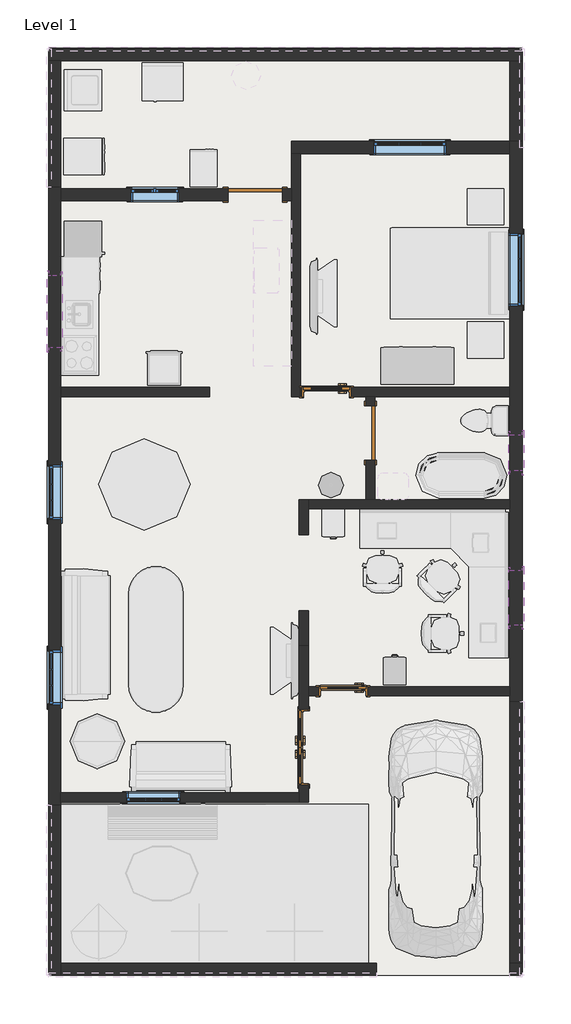
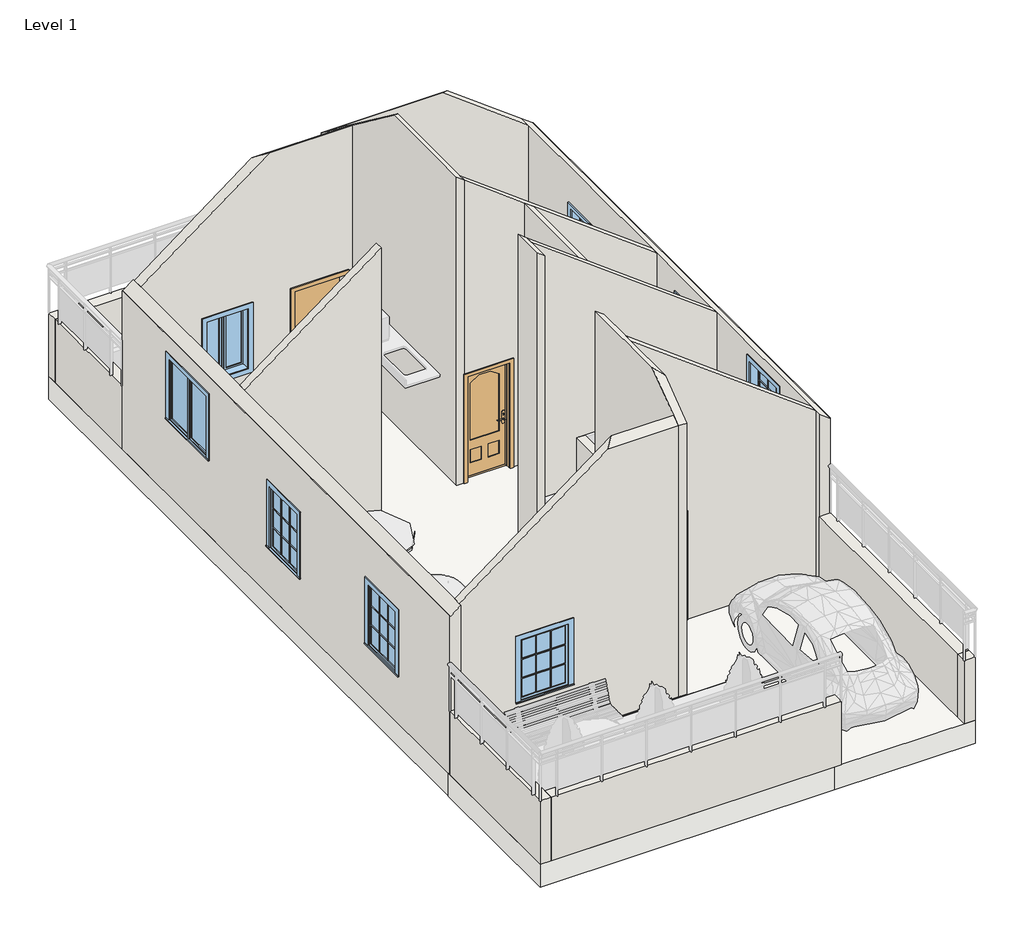
# One storey, part 1 of 3: 21 walls, 9 windows, 5 doors, 2 slabs.
"""IFC4 building model written with IfcOpenShell, lengths in millimetres."""

from ifc_helpers import new_model, si_unit, frame, origin, origin_with_axes, place, context, project, spatial, polyline, outline, extrude, faceted_brep, transform, mapped, element, save
from components import door_14b9be53, door_3efe7946, door_686f89d2, door_54dd4da4, window_29c06734, window_5c190c7e, window_99fc0ff6, window_bb17773d, window_0862ab64, window_e41d21a6

model = new_model("IFC4")

# Units and contexts
model_context = context("Model", 3, world=origin())
ifc_project = project(units=[si_unit("LENGTHUNIT", "METRE", prefix="MILLI")], contexts=[model_context])

# Site, building, storey
site = spatial("IfcSite", under=ifc_project)
building = spatial("IfcBuilding", under=site)
storey = spatial("IfcBuildingStorey", under=building, Name="Level 1", Elevation=0.0)

# Doors
placement = place(None, origin())
door_shape = door_14b9be53(model_context)
element("IfcDoor", 1, ObjectType="30\" x 80\"", at=placement, inside=storey, context=model_context, shape_type="MappedRepresentation", body=[
    mapped(door_shape, transform((-3257.4124913, 1119.1144299, 0.0), x_axis=(1.0, 0.0, 0.0), y_axis=(0.0, 1.0, 0.0), z_axis=(0.0, 0.0, 1.0))),
])
element("IfcDoor", 2, ObjectType="30\" x 80\"", at=placement, inside=storey, context=model_context, shape_type="MappedRepresentation", body=[
    mapped(door_shape, transform((-3536.8124913, 6122.9144299, 0.0), x_axis=(1.0, 0.0, 0.0), y_axis=(0.0, 1.0, 0.0), z_axis=(0.0, 0.0, 1.0))),
])
door_2_shape = door_3efe7946(model_context)
element("IfcDoor", 3, ObjectType="Door-Exterior-Double-Full Glass-Wood_Clad : 48\" x 80\"", at=placement, inside=storey, context=model_context, shape_type="MappedRepresentation", body=[
    mapped(door_2_shape, transform((-3920.9874913, 176.1394299, 0.0), x_axis=(0.0, 1.0, 0.0), y_axis=(-1.0, 0.0, 0.0), z_axis=(0.0, 0.0, 1.0))),
])
door_3_shape = door_686f89d2(model_context)
element("IfcDoor", 4, ObjectType="Single-Flush : 36\" x 84\"", at=placement, inside=storey, context=model_context, shape_type="MappedRepresentation", body=[
    mapped(door_3_shape, transform((-2800.2124913, 5433.9394299, 0.0), x_axis=(0.0, 1.0, 0.0), y_axis=(-1.0, 0.0, 0.0), z_axis=(0.0, 0.0, 1.0))),
])
door_4_shape = door_54dd4da4(model_context)
element("IfcDoor", 5, ObjectType="Single-Flush : 36\" x 84\"", at=placement, inside=storey, context=model_context, shape_type="MappedRepresentation", body=[
    mapped(door_4_shape, transform((-4730.6124913, 9421.7394299, 0.0), x_axis=(1.0, 0.0, 0.0), y_axis=(0.0, 1.0, 0.0), z_axis=(0.0, 0.0, 1.0))),
])

# Slabs
element("IfcSlab", 6, ObjectType="Steel Bar Joist 14\" - VCT on Concrete", at=placement, inside=storey, context=model_context, shape_type="SweptSolid", body=[
    extrude(outline(polyline([(-260.2124913, 11866.4894299), (-260.2124913, -3633.8605701), (-2825.6124913, -3633.8605701), (-2825.6124913, -763.6605701), (-8185.0124913, -763.6605701), (-8185.0124913, 11866.4894299), (-260.2124913, 11866.4894299)])), frame((0.0, 0.0, -441.325), z_axis=(0.0, 0.0, 1.0), x_axis=(1.0, 0.0, 0.0)), (0.0, 0.0, 1.0), 441.325),
])
element("IfcSlab", 7, ObjectType="Steel Bar Joist 14\" - VCT on Concrete", at=placement, inside=storey, context=model_context, shape_type="SweptSolid", body=[
    extrude(outline(polyline([(-8185.0124913, -738.2605701), (-7981.8124913, -738.2605701), (-7981.8124913, -3430.6605701), (-2825.6124913, -3430.6605701), (-2825.6124913, -3633.8605701), (-8185.0124913, -3633.8605701), (-8185.0124913, -738.2605701)])), frame((0.0, 0.0, -441.325), z_axis=(0.0, 0.0, 1.0), x_axis=(1.0, 0.0, 0.0)), (0.0, 0.0, 1.0), 441.325),
])

# Walls
element("IfcWall", 8, ObjectType="Generic - 8\"", at=placement, inside=storey, context=model_context, shape_type="Brep", body=[
    faceted_brep([(-8185.0124913, 11656.9394299, 0.0), (-7981.8124913, 11656.9394299, 0.0), (-463.4124913, 11656.9394299, 0.0), (-260.2124913, 11656.9394299, 0.0), (-260.2124913, 11656.9394299, 1219.2), (-463.4124913, 11656.9394299, 1219.2), (-7981.8124913, 11656.9394299, 1219.2), (-8185.0124913, 11656.9394299, 1219.2), (-8185.0124913, 11860.1394299, 0.0), (-8185.0124913, 11860.1394299, 1219.2), (-260.2124913, 11860.1394299, 1219.2), (-260.2124913, 11860.1394299, 0.0)], [[[0, 1, 2, 3, 4, 5, 6, 7]], [[8, 9, 10, 11]], [[3, 2, 1, 0, 8, 11]], [[7, 6, 5, 4, 10, 9]], [[0, 7, 9, 8]], [[4, 3, 11, 10]]]),
])
element("IfcWall", 9, ObjectType="Generic - 8\"", at=placement, inside=storey, context=model_context, shape_type="SweptSolid", body=[
    extrude(outline(polyline([(-8185.0124913, 9548.7394299), (-8185.0124913, 11656.9394299), (-7981.8124913, 11656.9394299), (-7981.8124913, 9548.7394299), (-8185.0124913, 9548.7394299)])), origin_with_axes(), (0.0, 0.0, 1.0), 1219.2),
])
element("IfcWall", 10, ObjectType="Generic - 8\"", at=placement, inside=storey, context=model_context, shape_type="SweptSolid", body=[
    extrude(outline(polyline([(-2698.6124913, -3633.8605701), (-7981.8124913, -3633.8605701), (-7981.8124913, -3430.6605701), (-2698.6124913, -3430.6605701), (-2698.6124913, -3633.8605701)])), origin_with_axes(), (0.0, 0.0, 1.0), 1219.2),
])
element("IfcWall", 11, ObjectType="Generic - 8\"", at=placement, inside=storey, context=model_context, shape_type="SweptSolid", body=[
    extrude(outline(polyline([(-260.2124913, 938.1394299), (-260.2124913, -3430.6605701), (-463.4124913, -3430.6605701), (-463.4124913, 938.1394299), (-260.2124913, 938.1394299)])), origin_with_axes(), (0.0, 0.0, 1.0), 1219.2),
])
element("IfcWall", 12, ObjectType="Generic - 8\"", at=placement, inside=storey, context=model_context, shape_type="Brep", body=[
    faceted_brep([(-463.4124913, 10310.7394299, 3193.25625), (-463.4124913, 10310.7394299, 0.0), (-4121.0124913, 10310.7394299, 0.0), (-4121.0124913, 10310.7394299, 4210.05), (-1819.1374913, 10310.7394299, 4210.05), (-1530.2124913, 10310.7394299, 1828.8), (-2749.4124913, 10310.7394299, 1828.8), (-2749.4124913, 10310.7394299, 304.8), (-1530.2124913, 10310.7394299, 304.8), (-463.4124913, 10107.5394299, 0.0), (-463.4124913, 10107.5394299, 3193.25625), (-2022.3374913, 10107.5394299, 4362.45), (-3968.6124913, 10107.5394299, 4362.45), (-4121.0124913, 10107.5394299, 4362.45), (-4121.0124913, 10107.5394299, 0.0), (-3968.6124913, 10107.5394299, 0.0), (-1530.2124913, 10107.5394299, 1828.8), (-1530.2124913, 10107.5394299, 304.8), (-2749.4124913, 10107.5394299, 304.8), (-2749.4124913, 10107.5394299, 1828.8)], [[[0, 1, 2, 3, 4], [5, 6, 7, 8]], [[9, 10, 11, 12, 13, 14, 15], [16, 17, 18, 19]], [[2, 1, 9, 15, 14]], [[3, 2, 14, 13]], [[0, 10, 9, 1]], [[0, 4, 11, 10]], [[4, 3, 13, 12, 11]], [[17, 16, 5, 8]], [[18, 17, 8, 7]], [[19, 18, 7, 6]], [[16, 19, 6, 5]]]),
])
element("IfcWall", 13, ObjectType="Generic - 8\"", at=placement, inside=storey, context=model_context, shape_type="Brep", body=[
    faceted_brep([(-4273.4124913, 9320.1394299, 2133.6), (-4273.4124913, 9320.1394299, 0.0), (-4121.0124913, 9320.1394299, 0.0), (-4121.0124913, 9320.1394299, 4953.0), (-5632.3124913, 9320.1394299, 4953.0), (-7981.8124913, 9320.1394299, 3190.875), (-7981.8124913, 9320.1394299, 0.0), (-5187.8124913, 9320.1394299, 0.0), (-5187.8124913, 9320.1394299, 2133.6), (-6000.6124913, 9320.1394299, 2133.6), (-6000.6124913, 9320.1394299, 914.4), (-6813.4124913, 9320.1394299, 914.4), (-6813.4124913, 9320.1394299, 2133.6), (-4121.0124913, 9523.3394299, 0.0), (-4273.4124913, 9523.3394299, 0.0), (-4273.4124913, 9523.3394299, 2133.6), (-5187.8124913, 9523.3394299, 2133.6), (-5187.8124913, 9523.3394299, 0.0), (-7981.8124913, 9523.3394299, 0.0), (-7981.8124913, 9523.3394299, 3190.875), (-5835.5124913, 9523.3394299, 4800.6), (-4121.0124913, 9523.3394299, 4800.6), (-6000.6124913, 9523.3394299, 2133.6), (-6813.4124913, 9523.3394299, 2133.6), (-6813.4124913, 9523.3394299, 914.4), (-6000.6124913, 9523.3394299, 914.4)], [[[0, 1, 2, 3, 4, 5, 6, 7, 8], [9, 10, 11, 12]], [[13, 14, 15, 16, 17, 18, 19, 20, 21], [22, 23, 24, 25]], [[7, 6, 18, 17]], [[2, 1, 14, 13]], [[6, 5, 19, 18]], [[3, 2, 13, 21]], [[5, 4, 20, 19]], [[4, 3, 21, 20]], [[15, 14, 1, 0]], [[16, 15, 0, 8]], [[17, 16, 8, 7]], [[10, 9, 22, 25]], [[11, 10, 25, 24]], [[12, 11, 24, 23]], [[9, 12, 23, 22]]]),
])
element("IfcWall", 14, ObjectType="Generic - 8\"", at=placement, inside=storey, context=model_context, shape_type="Brep", body=[
    faceted_brep([(-8185.0124913, -789.0605701, 0.0), (-8185.0124913, -3633.8605701, 0.0), (-8185.0124913, -3633.8605701, 1219.2), (-8185.0124913, -789.0605701, 1219.2), (-7981.8124913, -789.0605701, 0.0), (-7981.8124913, -789.0605701, 1219.2), (-7981.8124913, -3430.6605701, 1219.2), (-7981.8124913, -3633.8605701, 1219.2), (-7981.8124913, -3633.8605701, 0.0), (-7981.8124913, -3430.6605701, 0.0)], [[[0, 1, 2, 3]], [[4, 5, 6, 7, 8, 9]], [[1, 0, 4, 9, 8]], [[3, 2, 7, 6, 5]], [[0, 3, 5, 4]], [[2, 1, 8, 7]]]),
])
element("IfcWall", 15, ObjectType="Generic - 8\"", at=placement, inside=storey, context=model_context, shape_type="SweptSolid", body=[
    extrude(outline(polyline([(-260.2124913, -3633.8605701), (-463.4124913, -3633.8605701), (-463.4124913, -3430.6605701), (-260.2124913, -3430.6605701), (-260.2124913, -3633.8605701)])), origin_with_axes(), (0.0, 0.0, 1.0), 1219.2),
])
element("IfcWall", 16, ObjectType="Generic - 8\"", at=placement, inside=storey, context=model_context, shape_type="Brep", body=[
    faceted_brep([(-260.2124913, 938.1394299, 0.0), (-260.2124913, 10310.7394299, 0.0), (-260.2124913, 10310.7394299, 1219.2), (-260.2124913, 10310.7394299, 3048.0), (-260.2124913, 938.1394299, 3048.0), (-260.2124913, 938.1394299, 1219.2), (-260.2124913, 2220.8394299, 2927.35), (-260.2124913, 3135.2394299, 2927.35), (-260.2124913, 3135.2394299, 1708.15), (-260.2124913, 2220.8394299, 1708.15), (-260.2124913, 7554.8394299, 2438.4), (-260.2124913, 8774.0394299, 2438.4), (-260.2124913, 8774.0394299, 914.4), (-260.2124913, 7554.8394299, 914.4), (-260.2124913, 4798.9394299, 2768.6), (-260.2124913, 5408.5394299, 2768.6), (-260.2124913, 5408.5394299, 2159.0), (-260.2124913, 4798.9394299, 2159.0), (-463.4124913, 938.1394299, 0.0), (-463.4124913, 938.1394299, 1219.2), (-463.4124913, 938.1394299, 3193.25625), (-463.4124913, 1039.7394299, 3193.25625), (-463.4124913, 1192.1394299, 3193.25625), (-463.4124913, 4163.9394299, 3193.25625), (-463.4124913, 4316.3394299, 3193.25625), (-463.4124913, 6043.5394299, 3193.25625), (-463.4124913, 6195.9394299, 3193.25625), (-463.4124913, 10107.5394299, 3193.25625), (-463.4124913, 10310.7394299, 3193.25625), (-463.4124913, 10310.7394299, 1219.2), (-463.4124913, 10310.7394299, 0.0), (-463.4124913, 10107.5394299, 0.0), (-463.4124913, 6195.9394299, 0.0), (-463.4124913, 6043.5394299, 0.0), (-463.4124913, 4316.3394299, 0.0), (-463.4124913, 4163.9394299, 0.0), (-463.4124913, 1192.1394299, 0.0), (-463.4124913, 1039.7394299, 0.0), (-463.4124913, 2220.8394299, 2927.35), (-463.4124913, 2220.8394299, 1708.15), (-463.4124913, 3135.2394299, 1708.15), (-463.4124913, 3135.2394299, 2927.35), (-463.4124913, 7554.8394299, 2438.4), (-463.4124913, 7554.8394299, 914.4), (-463.4124913, 8774.0394299, 914.4), (-463.4124913, 8774.0394299, 2438.4), (-463.4124913, 4798.9394299, 2768.6), (-463.4124913, 4798.9394299, 2159.0), (-463.4124913, 5408.5394299, 2159.0), (-463.4124913, 5408.5394299, 2768.6), (-269.7374913, 938.1394299, 3048.0), (-269.7374913, 10310.7394299, 3048.0)], [[[0, 1, 2, 3, 4, 5], [6, 7, 8, 9], [10, 11, 12, 13], [14, 15, 16, 17]], [[18, 19, 20, 21, 22, 23, 24, 25, 26, 27, 28, 29, 30, 31, 32, 33, 34, 35, 36, 37], [38, 39, 40, 41], [42, 43, 44, 45], [46, 47, 48, 49]], [[1, 0, 18, 37, 36, 35, 34, 33, 32, 31, 30]], [[0, 5, 4, 50, 20, 19, 18]], [[1, 30, 29, 28, 51, 3, 2]], [[4, 3, 51, 50]], [[51, 28, 27, 26, 25, 24, 23, 22, 21, 20, 50]], [[39, 38, 6, 9]], [[40, 39, 9, 8]], [[41, 40, 8, 7]], [[38, 41, 7, 6]], [[43, 42, 10, 13]], [[44, 43, 13, 12]], [[45, 44, 12, 11]], [[42, 45, 11, 10]], [[47, 46, 14, 17]], [[48, 47, 17, 16]], [[49, 48, 16, 15]], [[46, 49, 15, 14]]]),
])
element("IfcWall", 17, ObjectType="Generic - 8\"", at=placement, inside=storey, context=model_context, shape_type="Brep", body=[
    faceted_brep([(-8185.0124913, 9548.7394299, 0.0), (-8185.0124913, -789.0605701, 0.0), (-8185.0124913, -789.0605701, 1219.2), (-8185.0124913, -789.0605701, 3048.0), (-8185.0124913, 9548.7394299, 3048.0), (-8185.0124913, 9548.7394299, 1219.2), (-8185.0124913, 1801.7394299, 2133.6), (-8185.0124913, 887.3394299, 2133.6), (-8185.0124913, 887.3394299, 914.4), (-8185.0124913, 1801.7394299, 914.4), (-8185.0124913, 4900.5394299, 2133.6), (-8185.0124913, 3986.1394299, 2133.6), (-8185.0124913, 3986.1394299, 914.4), (-8185.0124913, 4900.5394299, 914.4), (-8185.0124913, 8075.5394299, 2667.0), (-8185.0124913, 6856.3394299, 2667.0), (-8185.0124913, 6856.3394299, 1447.8), (-8185.0124913, 8075.5394299, 1447.8), (-7981.8124913, 9548.7394299, 0.0), (-7981.8124913, 9548.7394299, 1219.2), (-7981.8124913, 9548.7394299, 3190.875), (-7981.8124913, 9523.3394299, 3190.875), (-7981.8124913, 9320.1394299, 3190.875), (-7981.8124913, 6195.9394299, 3190.875), (-7981.8124913, 6043.5394299, 3190.875), (-7981.8124913, -585.8605701, 3190.875), (-7981.8124913, -738.2605701, 3190.875), (-7981.8124913, -789.0605701, 3190.875), (-7981.8124913, -789.0605701, 1219.2), (-7981.8124913, -789.0605701, 0.0), (-7981.8124913, -738.2605701, 0.0), (-7981.8124913, -585.8605701, 0.0), (-7981.8124913, 6043.5394299, 0.0), (-7981.8124913, 6195.9394299, 0.0), (-7981.8124913, 9320.1394299, 0.0), (-7981.8124913, 9523.3394299, 0.0), (-7981.8124913, 1801.7394299, 2133.6), (-7981.8124913, 1801.7394299, 914.4), (-7981.8124913, 887.3394299, 914.4), (-7981.8124913, 887.3394299, 2133.6), (-7981.8124913, 4900.5394299, 2133.6), (-7981.8124913, 4900.5394299, 914.4), (-7981.8124913, 3986.1394299, 914.4), (-7981.8124913, 3986.1394299, 2133.6), (-7981.8124913, 8075.5394299, 2667.0), (-7981.8124913, 8075.5394299, 1447.8), (-7981.8124913, 6856.3394299, 1447.8), (-7981.8124913, 6856.3394299, 2667.0), (-8172.3124913, -789.0605701, 3048.0), (-8172.3124913, 9548.7394299, 3048.0)], [[[0, 1, 2, 3, 4, 5], [6, 7, 8, 9], [10, 11, 12, 13], [14, 15, 16, 17]], [[18, 19, 20, 21, 22, 23, 24, 25, 26, 27, 28, 29, 30, 31, 32, 33, 34, 35], [36, 37, 38, 39], [40, 41, 42, 43], [44, 45, 46, 47]], [[1, 0, 18, 35, 34, 33, 32, 31, 30, 29]], [[3, 2, 1, 29, 28, 27, 48]], [[0, 5, 4, 49, 20, 19, 18]], [[4, 3, 48, 49]], [[48, 27, 26, 25, 24, 23, 22, 21, 20, 49]], [[37, 36, 6, 9]], [[38, 37, 9, 8]], [[39, 38, 8, 7]], [[36, 39, 7, 6]], [[41, 40, 10, 13]], [[42, 41, 13, 12]], [[43, 42, 12, 11]], [[40, 43, 11, 10]], [[45, 44, 14, 17]], [[46, 45, 17, 16]], [[47, 46, 16, 15]], [[44, 47, 15, 14]]]),
])
element("IfcWall", 18, ObjectType="Generic - 8\"", at=placement, inside=storey, context=model_context, shape_type="SweptSolid", body=[
    extrude(outline(polyline([(-260.2124913, 11656.9394299), (-260.2124913, 10310.7394299), (-463.4124913, 10310.7394299), (-463.4124913, 11656.9394299), (-260.2124913, 11656.9394299)])), origin_with_axes(), (0.0, 0.0, 1.0), 1219.2),
])
element("IfcWall", 19, ObjectType="INNER WALL", at=placement, inside=storey, context=model_context, shape_type="Brep", body=[
    faceted_brep([(-4121.0124913, 10107.5394299, 0.0), (-4121.0124913, 9523.3394299, 0.0), (-4121.0124913, 9320.1394299, 0.0), (-4121.0124913, 6043.5394299, 0.0), (-4121.0124913, 6043.5394299, 5936.45625), (-4121.0124913, 8008.8644299, 5936.45625), (-4121.0124913, 9320.1394299, 4953.0), (-4121.0124913, 9523.3394299, 4800.6), (-4121.0124913, 10107.5394299, 4362.45), (-3968.6124913, 10107.5394299, 0.0), (-3968.6124913, 10107.5394299, 4362.45), (-3968.6124913, 8161.2644299, 5822.15625), (-3968.6124913, 6195.9394299, 5822.15625), (-3968.6124913, 6043.5394299, 5822.15625), (-3968.6124913, 6043.5394299, 0.0), (-3968.6124913, 6195.9394299, 0.0)], [[[0, 1, 2, 3, 4, 5, 6, 7, 8]], [[9, 10, 11, 12, 13, 14, 15]], [[3, 2, 1, 0, 9, 15, 14]], [[0, 8, 10, 9]], [[4, 3, 14, 13]], [[8, 7, 6, 5, 11, 10]], [[5, 4, 13, 12, 11]]]),
])
element("IfcWall", 20, ObjectType="INNER WALL", at=placement, inside=storey, context=model_context, shape_type="Brep", body=[
    faceted_brep([(-463.4124913, 6195.9394299, 3193.25625), (-463.4124913, 6195.9394299, 0.0), (-3130.4124913, 6195.9394299, 0.0), (-3130.4124913, 6195.9394299, 2057.4), (-3943.2124913, 6195.9394299, 2057.4), (-3943.2124913, 6195.9394299, 0.0), (-3968.6124913, 6195.9394299, 0.0), (-3968.6124913, 6195.9394299, 5822.15625), (-463.4124913, 6043.5394299, 0.0), (-463.4124913, 6043.5394299, 3193.25625), (-2724.0124913, 6043.5394299, 4888.70625), (-2876.4124913, 6043.5394299, 5003.00625), (-3968.6124913, 6043.5394299, 5822.15625), (-3968.6124913, 6043.5394299, 0.0), (-3943.2124913, 6043.5394299, 0.0), (-3943.2124913, 6043.5394299, 2057.4), (-3130.4124913, 6043.5394299, 2057.4), (-3130.4124913, 6043.5394299, 0.0), (-2876.4124913, 6043.5394299, 0.0), (-2724.0124913, 6043.5394299, 0.0)], [[[0, 1, 2, 3, 4, 5, 6, 7]], [[8, 9, 10, 11, 12, 13, 14, 15, 16, 17, 18, 19]], [[1, 8, 19, 18, 17, 2]], [[13, 6, 5, 14]], [[1, 0, 9, 8]], [[7, 6, 13, 12]], [[0, 7, 12, 11, 10, 9]], [[16, 3, 2, 17]], [[3, 16, 15, 4]], [[4, 15, 14, 5]]]),
])
element("IfcWall", 21, ObjectType="INNER WALL", at=placement, inside=storey, context=model_context, shape_type="Brep", body=[
    faceted_brep([(-463.4124913, 4316.3394299, 0.0), (-2724.0124913, 4316.3394299, 0.0), (-2876.4124913, 4316.3394299, 0.0), (-3841.6124913, 4316.3394299, 0.0), (-3841.6124913, 4316.3394299, 5726.90625), (-2876.4124913, 4316.3394299, 5003.00625), (-2724.0124913, 4316.3394299, 4888.70625), (-463.4124913, 4316.3394299, 3193.25625), (-463.4124913, 4163.9394299, 0.0), (-463.4124913, 4163.9394299, 3193.25625), (-3841.6124913, 4163.9394299, 5726.90625), (-3841.6124913, 4163.9394299, 0.0)], [[[0, 1, 2, 3, 4, 5, 6, 7]], [[8, 9, 10, 11]], [[3, 2, 1, 0, 8, 11]], [[0, 7, 9, 8]], [[4, 3, 11, 10]], [[7, 6, 5, 4, 10, 9]]]),
])
element("IfcWall", 22, ObjectType="INNER WALL", at=placement, inside=storey, context=model_context, shape_type="SweptSolid", body=[
    extrude(outline(polyline([(0.0, -463.4124913), (3193.25625, -463.4124913), (5726.90625, -3841.6124913), (0.0, -3841.6124913), (0.0, -3663.8124913), (2057.4, -3663.8124913), (2057.4, -2851.0124913), (0.0, -2851.0124913), (0.0, -463.4124913)])), frame((0.0, 1039.7394299, 0.0), z_axis=(0.0, 1.0, 0.0), x_axis=(0.0, 0.0, 1.0)), (0.0, 0.0, 1.0), 152.4),
])
element("IfcWall", 23, ObjectType="INNER WALL", at=placement, inside=storey, context=model_context, shape_type="Brep", body=[
    faceted_brep([(-3994.0124913, -585.8605701, 0.0), (-7981.8124913, -585.8605701, 0.0), (-7981.8124913, -585.8605701, 3190.875), (-5127.4874913, -585.8605701, 5331.61875), (-3994.0124913, -585.8605701, 5331.61875), (-6889.6124913, -585.8605701, 2133.6), (-6889.6124913, -585.8605701, 914.4), (-5975.2124913, -585.8605701, 914.4), (-5975.2124913, -585.8605701, 2133.6), (-3994.0124913, -738.2605701, 0.0), (-3994.0124913, -738.2605701, 5217.31875), (-5279.8874913, -738.2605701, 5217.31875), (-7981.8124913, -738.2605701, 3190.875), (-7981.8124913, -738.2605701, 0.0), (-6889.6124913, -738.2605701, 2133.6), (-5975.2124913, -738.2605701, 2133.6), (-5975.2124913, -738.2605701, 914.4), (-6889.6124913, -738.2605701, 914.4)], [[[0, 1, 2, 3, 4], [5, 6, 7, 8]], [[9, 10, 11, 12, 13], [14, 15, 16, 17]], [[1, 0, 9, 13]], [[2, 1, 13, 12]], [[0, 4, 10, 9]], [[4, 3, 11, 10]], [[3, 2, 12, 11]], [[6, 5, 14, 17]], [[7, 6, 17, 16]], [[8, 7, 16, 15]], [[5, 8, 15, 14]]]),
])
element("IfcWall", 24, ObjectType="INNER WALL", at=placement, inside=storey, context=model_context, shape_type="SweptSolid", body=[
    extrude(outline(polyline([(0.0, -5492.6124913), (5057.775, -5492.6124913), (3190.875, -7981.8124913), (0.0, -7981.8124913), (0.0, -5492.6124913)])), frame((0.0, 6043.5394299, 0.0), z_axis=(0.0, 1.0, 0.0), x_axis=(0.0, 0.0, 1.0)), (0.0, 0.0, 1.0), 152.4),
])
element("IfcWall", 25, ObjectType="INNER WALL", at=placement, inside=storey, context=model_context, shape_type="Brep", body=[
    faceted_brep([(-3994.0124913, 1877.9394299, 5841.20625), (-3994.0124913, 1877.9394299, 3048.0), (-3994.0124913, 1877.9394299, 0.0), (-3994.0124913, 811.1394299, 0.0), (-3994.0124913, 811.1394299, 2057.4), (-3994.0124913, -458.8605701, 2057.4), (-3994.0124913, -458.8605701, 0.0), (-3994.0124913, -585.8605701, 0.0), (-3994.0124913, -738.2605701, 0.0), (-3994.0124913, -738.2605701, 5217.31875), (-3994.0124913, -585.8605701, 5331.61875), (-3994.0124913, 93.5894299, 5841.20625), (-3841.6124913, 1877.9394299, 0.0), (-3841.6124913, 1877.9394299, 3048.0), (-3841.6124913, 1877.9394299, 5726.90625), (-3841.6124913, 1192.1394299, 5726.90625), (-3841.6124913, 1039.7394299, 5726.90625), (-3841.6124913, -58.8105701, 5726.90625), (-3841.6124913, -738.2605701, 5217.31875), (-3841.6124913, -738.2605701, 0.0), (-3841.6124913, -458.8605701, 0.0), (-3841.6124913, -458.8605701, 2057.4), (-3841.6124913, 811.1394299, 2057.4), (-3841.6124913, 811.1394299, 0.0), (-3841.6124913, 1039.7394299, 0.0), (-3841.6124913, 1192.1394299, 0.0)], [[[0, 1, 2, 3, 4, 5, 6, 7, 8, 9, 10, 11]], [[12, 13, 14, 15, 16, 17, 18, 19, 20, 21, 22, 23, 24, 25]], [[19, 8, 7, 6, 20]], [[2, 12, 25, 24, 23, 3]], [[2, 1, 0, 14, 13, 12]], [[9, 8, 19, 18]], [[14, 0, 11, 17, 16, 15]], [[9, 18, 17, 11, 10]], [[22, 4, 3, 23]], [[4, 22, 21, 5]], [[5, 21, 20, 6]]]),
])
element("IfcWall", 26, ObjectType="INNER WALL", at=placement, inside=storey, context=model_context, shape_type="Brep", body=[
    faceted_brep([(-2876.4124913, 6043.5394299, 0.0), (-2876.4124913, 5891.1394299, 0.0), (-2876.4124913, 5891.1394299, 2133.6), (-2876.4124913, 4976.7394299, 2133.6), (-2876.4124913, 4976.7394299, 0.0), (-2876.4124913, 4316.3394299, 0.0), (-2876.4124913, 4316.3394299, 5003.00625), (-2876.4124913, 6043.5394299, 5003.00625), (-2724.0124913, 5891.1394299, 2133.6), (-2724.0124913, 5891.1394299, 0.0), (-2724.0124913, 6043.5394299, 0.0), (-2724.0124913, 6043.5394299, 4888.70625), (-2724.0124913, 4316.3394299, 4888.70625), (-2724.0124913, 4316.3394299, 0.0), (-2724.0124913, 4976.7394299, 0.0), (-2724.0124913, 4976.7394299, 2133.6)], [[[0, 1, 2, 3, 4, 5, 6, 7]], [[8, 9, 10, 11, 12, 13, 14, 15]], [[14, 13, 5, 4]], [[10, 9, 1, 0]], [[0, 7, 11, 10]], [[6, 5, 13, 12]], [[7, 6, 12, 11]], [[2, 1, 9, 8]], [[3, 2, 8, 15]], [[4, 3, 15, 14]]]),
])
element("IfcWall", 27, ObjectType="INNER WALL", at=placement, inside=storey, context=model_context, shape_type="Brep", body=[
    faceted_brep([(-3994.0124913, 4316.3394299, 0.0), (-3994.0124913, 3732.1394299, 0.0), (-3994.0124913, 3732.1394299, 5841.20625), (-3994.0124913, 4316.3394299, 5841.20625), (-3841.6124913, 4316.3394299, 0.0), (-3841.6124913, 4316.3394299, 5726.90625), (-3841.6124913, 4163.9394299, 5726.90625), (-3841.6124913, 3732.1394299, 5726.90625), (-3841.6124913, 3732.1394299, 0.0), (-3841.6124913, 4163.9394299, 0.0)], [[[0, 1, 2, 3]], [[4, 5, 6, 7, 8, 9]], [[1, 0, 4, 9, 8]], [[2, 1, 8, 7]], [[0, 3, 5, 4]], [[3, 2, 7, 6, 5]]]),
])
element("IfcWall", 28, ObjectType="INNER WALL", at=placement, inside=storey, context=model_context, shape_type="SweptSolid", body=[
    extrude(outline(polyline([(-3841.6124913, 2462.1394299), (-3841.6124913, 1877.9394299), (-3994.0124913, 1877.9394299), (-3994.0124913, 2462.1394299), (-3841.6124913, 2462.1394299)])), origin_with_axes(), (0.0, 0.0, 1.0), 3048.0),
])

# Windows
window_shape = window_29c06734(model_context)
element("IfcWindow", 29, ObjectType="Casement 3x3 with Trim : 36\" x 48\"", at=placement, inside=storey, context=model_context, shape_type="MappedRepresentation", body=[
    mapped(window_shape, transform((-361.8124913, 2678.0394299, 793.75), x_axis=(0.0, -1.0, 0.0), y_axis=(1.0, 0.0, 0.0), z_axis=(0.0, 0.0, 1.0))),
])
element("IfcWindow", 30, ObjectType="Casement 3x3 with Trim : 36\" x 48\"", at=placement, inside=storey, context=model_context, shape_type="MappedRepresentation", body=[
    mapped(window_shape, transform((-8083.4124913, 1344.5394299, 0.0), x_axis=(0.0, 1.0, 0.0), y_axis=(-1.0, 0.0, 0.0), z_axis=(0.0, 0.0, 1.0))),
])
element("IfcWindow", 31, ObjectType="Casement 3x3 with Trim : 36\" x 48\"", at=placement, inside=storey, context=model_context, shape_type="MappedRepresentation", body=[
    mapped(window_shape, transform((-8083.4124913, 4443.3394299, 0.0), x_axis=(0.0, 1.0, 0.0), y_axis=(-1.0, 0.0, 0.0), z_axis=(0.0, 0.0, 1.0))),
])
window_2_shape = window_5c190c7e(model_context)
element("IfcWindow", 32, ObjectType="Casement 3x3 with Trim : 36\" x 48\"", at=placement, inside=storey, context=model_context, shape_type="MappedRepresentation", body=[
    mapped(window_2_shape, transform((-6432.4124913, -662.0605701, 0.0), x_axis=(-1.0, 0.0, 0.0), y_axis=(0.0, -1.0, 0.0), z_axis=(0.0, 0.0, 1.0))),
])
window_3_shape = window_99fc0ff6(model_context)
element("IfcWindow", 33, ObjectType="Casement 3x3 with Trim : 48\" x 60\"", at=placement, inside=storey, context=model_context, shape_type="MappedRepresentation", body=[
    mapped(window_3_shape, transform((-361.8124913, 8164.4394299, 609.6), x_axis=(0.0, -1.0, 0.0), y_axis=(1.0, 0.0, 0.0), z_axis=(0.0, 0.0, 1.0))),
])
element("IfcWindow", 34, ObjectType="Casement 3x3 with Trim : 48\" x 60\"", at=placement, inside=storey, context=model_context, shape_type="MappedRepresentation", body=[
    mapped(window_3_shape, transform((-2139.8124913, 10209.1394299, 0.0), x_axis=(1.0, 0.0, 0.0), y_axis=(0.0, 1.0, 0.0), z_axis=(0.0, 0.0, 1.0))),
])
window_4_shape = window_bb17773d(model_context)
element("IfcWindow", 35, ObjectType="Casement Dbl with Trim : 32\" x 48\"", at=placement, inside=storey, context=model_context, shape_type="MappedRepresentation", body=[
    mapped(window_4_shape, transform((-6407.0124913, 9402.6894299, 0.0), x_axis=(1.0, 0.0, 0.0), y_axis=(0.0, 1.0, 0.0), z_axis=(0.0, 0.0, 1.0))),
])
window_5_shape = window_0862ab64(model_context)
element("IfcWindow", 36, ObjectType="Casement Dbl with Trim : 48\" x 48\"", at=placement, inside=storey, context=model_context, shape_type="MappedRepresentation", body=[
    mapped(window_5_shape, transform((-8064.3624913, 7465.9394299, 533.4), x_axis=(0.0, 1.0, 0.0), y_axis=(-1.0, 0.0, 0.0), z_axis=(0.0, 0.0, 1.0))),
])
window_6_shape = window_e41d21a6(model_context)
element("IfcWindow", 37, ObjectType="Transom with Trim : 24\" x 24\"", at=placement, inside=storey, context=model_context, shape_type="MappedRepresentation", body=[
    mapped(window_6_shape, transform((-361.8124913, 5065.6394299, 0.0), x_axis=(0.0, -1.0, 0.0), y_axis=(1.0, 0.0, 0.0), z_axis=(0.0, 0.0, 1.0))),
])

save(model, "model.ifc")

# Revit data of these elements
# Type "30\" x 80\""
#   Type Mark = "9"
#   Assembly Code = "B2030100"
#   Analytic Construction = "French door, wood frame with single glass"
#   Threshold Offset [instance default] = 0' - 0 1/2"
#   Thickness = 0' - 1 3/8"
#   Thermal Resistance (R) = 1.0696 (h·ft²·°F)/BTU
#   Swing Angle [instance default] = 90.00°
#   Stiles = 0' - 4 3/4"
#   Rough Width = 2' - 8"
#   Rough Height = 6' - 9"
#   Radius = 1' - 1.00625"
#   Lock Rail = 0' - 7 1/8"
#   Height = 6' - 8"
#   Width = 2' - 6"
#   Heat Transfer Coefficient (U) = 0.9350 BTU/(h·ft²·°F)
#   Door Offset [instance default] = 0' - 0"
#   Bottom Rail = 0' - 9 1/2"
#   Threshold [instance default] = yes
#   Function = 1
#   Exterior Trim [instance default] = yes
#   Trim Material = Cherry
#   Threshold Material = Cherry
#   Panel Material = Cherry
#   Glazing = Glass
#   Frame Material = Cherry
#   Door Handle Material = Aluminum
#   Visual Light Transmittance = 0
#   Solar Heat Gain Coefficient = 0
#   Wall Closure = (empty or 0)
#   Construction Type = (empty or 0)
# Type "Door-Exterior-Double-Full Glass-Wood_Clad : 48\" x 80\""
#   Type Mark = "8"
#   Assembly Code = "B2030100"
#   Analytic Construction = "French door, wood frame with double glass"
#   Top Rail = 0' - 4 11/16"
#   Threshold Offset [instance default] = 0' - 0 1/2"
#   Thickness = 0' - 1 3/8"
#   Thermal Resistance (R) = 1.9158 (h·ft²·°F)/BTU
#   Swing Angle [instance default] = 90.00°
#   Stiles = 0' - 4 3/4"
#   Rough Width = 4' - 2"
#   Rough Height = 6' - 9"
#   Panel Width = 2' - 0"
#   Door Offset [instance default] = 0' - 0"
#   Height = 6' - 8"
#   Width = 4' - 0"
#   Heat Transfer Coefficient (U) = 0.5220 BTU/(h·ft²·°F)
#   Bottom Rail = 0' - 9 1/8"
#   Exterior Trim [instance default] = yes
#   Threshold [instance default] = yes
#   Show Grill [instance default] = yes
#   Function = 1
#   Trim Material = Cherry
#   Threshold Material = Cherry
#   Panel Material = Cherry
#   Glazing = Glass
#   Frame Material = Cherry
#   Door Handle Material = Aluminum
#   Visual Light Transmittance = 0
#   Solar Heat Gain Coefficient = 0
#   Wall Closure = (empty or 0)
#   Construction Type = (empty or 0)
# Type "Single-Flush : 36\" x 84\""
#   Type Mark = "1"
#   Construction Type Id = "MDOOR"
#   Assembly Code = "C1020"
#   Analytic Construction = "Metal"
#   Thickness = 0' - 2"
#   Heat Transfer Coefficient (U) = 0.651978 BTU/(h·ft²·°F)
#   Height = 7' - 0"
#   Trim Projection Ext = 0' - 1"
#   Trim Projection Int = 0' - 1"
#   Trim Width = 0' - 3"
#   Width = 3' - 0"
#   Define Thermal Properties by = 1
#   Door Material = Door - Panel
#   Frame Material = Door - Frame
#   Visual Light Transmittance = 0
#   Solar Heat Gain Coefficient = 0
#   Function = (empty or 0)
#   Wall Closure = (empty or 0)
# Type "Steel Bar Joist 14\" - VCT on Concrete"
#   Assembly Code = "B1010"
#   Function = 0
#   Layers, outside or top first: 0' - 0 1/4" "Vinyl Composition Tile" (function 5); 0' - 3" "Concrete, Lightweight" (function 1); 0' - 0 1/8" "Metal Deck" (function 1); 1' - 2" "Structure, Steel Bar Joist Layer" (function 1)
# Type "Generic - 8\""
#   Assembly Code = "B2010"
#   Layers, outside or top first: 0' - 8" "Brick, Common" (function 1)
# Type "INNER WALL"
#   Assembly Code = "B2010"
#   Layers, outside or top first: 0' - 6" "Brick, Soldier Course" (function 1)
# Type "Casement 3x3 with Trim : 36\" x 48\""
#   Type Mark = "10"
#   Construction Type Id = "GSP4R"
#   Assembly Code = "B2020100"
#   Analytic Construction = "1/8 in Pilkington single glazing"
#   Visual Light Transmittance = 0.9
#   Solar Heat Gain Coefficient = 0.78
#   Heat Transfer Coefficient (U) = 0.6496 BTU/(h·ft²·°F)
#   Height = 4' - 0"
#   Default Sill Height = 3' - 0"
#   Trim Projection - Ext. = 0' - 0 1/2"
#   Trim Projection - Int. = 0' - 0 3/4"
#   Trim Width - Exterior = 0' - 3 1/2"
#   Trim Width - Interior = 0' - 3 1/2"
#   Width = 3' - 0"
#   Window Inset = 0' - 0 3/4"
#   Define Thermal Properties by = 1
#   Glass Pane Material = Glass
#   Sash Material = Sash
#   Trim Exterior Material = Trim
#   Trim Interior Material = Trim
#   Wall Closure = (empty or 0)
# Type "Casement 3x3 with Trim : 48\" x 60\""
#   Type Mark = "12"
#   Construction Type Id = "GSP4R"
#   Assembly Code = "B2020100"
#   Analytic Construction = "1/8 in Pilkington single glazing"
#   Visual Light Transmittance = 0.9
#   Solar Heat Gain Coefficient = 0.78
#   Heat Transfer Coefficient (U) = 0.6496 BTU/(h·ft²·°F)
#   Height = 5' - 0"
#   Default Sill Height = 1' - 0"
#   Trim Projection - Ext. = 0' - 0 1/2"
#   Trim Projection - Int. = 0' - 0 3/4"
#   Trim Width - Exterior = 0' - 3 1/2"
#   Trim Width - Interior = 0' - 3 1/2"
#   Width = 4' - 0"
#   Window Inset = 0' - 0 3/4"
#   Define Thermal Properties by = 1
#   Glass Pane Material = Glass
#   Sash Material = Sash
#   Trim Exterior Material = Trim
#   Trim Interior Material = Trim
#   Wall Closure = (empty or 0)
# Type "Casement Dbl with Trim : 32\" x 48\""
#   Type Mark = "15"
#   Construction Type Id = "GSP4R"
#   Assembly Code = "B2020100"
#   Analytic Construction = "1/8 in Pilkington single glazing"
#   Visual Light Transmittance = 0.9
#   Solar Heat Gain Coefficient = 0.78
#   Heat Transfer Coefficient (U) = 0.6496 BTU/(h·ft²·°F)
#   Height = 4' - 0"
#   Default Sill Height = 3' - 0"
#   Trim Projection - Ext. = 0' - 0 1/2"
#   Trim Projection - Int. = 0' - 0 3/4"
#   Trim Width - Exterior = 0' - 3 1/2"
#   Trim Width - Interior = 0' - 3 1/2"
#   Width = 2' - 8"
#   Window Inset = 0' - 0 3/4"
#   Define Thermal Properties by = 1
#   Glass Pane Material = Glass
#   Sash Material = Sash
#   Trim Exterior Material = Trim
#   Trim Interior Material = Trim
#   Wall Closure = (empty or 0)
# Type "Casement Dbl with Trim : 48\" x 48\""
#   Type Mark = "13"
#   Construction Type Id = "GSP4R"
#   Assembly Code = "B2020100"
#   Analytic Construction = "1/8 in Pilkington single glazing"
#   Visual Light Transmittance = 0.9
#   Solar Heat Gain Coefficient = 0.78
#   Heat Transfer Coefficient (U) = 0.6496 BTU/(h·ft²·°F)
#   Height = 4' - 0"
#   Default Sill Height = 3' - 0"
#   Trim Projection - Ext. = 0' - 0 1/2"
#   Trim Projection - Int. = 0' - 0 3/4"
#   Trim Width - Exterior = 0' - 3 1/2"
#   Trim Width - Interior = 0' - 3 1/2"
#   Width = 4' - 0"
#   Window Inset = 0' - 0 3/4"
#   Define Thermal Properties by = 1
#   Glass Pane Material = Glass
#   Sash Material = Sash
#   Trim Exterior Material = Trim
#   Trim Interior Material = Trim
#   Wall Closure = (empty or 0)
# Type "Transom with Trim : 24\" x 24\""
#   Type Mark = "16"
#   Construction Type Id = "GSP4R"
#   Assembly Code = "B2020100"
#   Analytic Construction = "1/8 in Pilkington single glazing"
#   Visual Light Transmittance = 0.9
#   Solar Heat Gain Coefficient = 0.78
#   Heat Transfer Coefficient (U) = 0.6496 BTU/(h·ft²·°F)
#   Height = 2' - 0"
#   Default Sill Height = 7' - 1"
#   Trim Projection - Ext. = 0' - 0 1/2"
#   Trim Projection - Int. = 0' - 0 3/4"
#   Trim Width - Exterior = 0' - 3 1/2"
#   Trim Width - Interior = 0' - 3 1/2"
#   Width = 2' - 0"
#   Window Inset = 0' - 0 3/4"
#   Define Thermal Properties by = 1
#   Glass Pane Material = Glass
#   Sash Material = Sash
#   Trim Exterior Material = Trim
#   Trim Interior Material = Trim
#   Wall Closure = (empty or 0)
# Elements 1, 2 (IfcDoor, "30\" x 80\"")
#   Threshold Offset = 0' - 0 1/2"
#   Swing Angle = 90.00°
#   Door Offset = 0' - 0"
#   Threshold = yes
#   Exterior Trim = yes
#   Phase Created = New Construction
#   Materials on its faces: "Cherry", "Aluminum", "Glass"
# Element 3 (IfcDoor, "Door-Exterior-Double-Full Glass-Wood_Clad : 48\" x 80\"")
#   Threshold Offset = 0' - 0 1/2"
#   Swing Angle = 90.00°
#   Door Offset = 0' - 0"
#   Threshold = yes
#   Show Grill = yes
#   Exterior Trim = yes
#   Phase Created = New Construction
#   Materials on its faces: "Cherry", "Aluminum", "Glass"
# Elements 4, 5 (IfcDoor, "Single-Flush : 36\" x 84\"")
#   Phase Created = New Construction
#   Materials on its faces: "Door - Frame", "Door - Panel"
# Element 6 (IfcSlab, "Steel Bar Joist 14\" - VCT on Concrete")
#   Height Offset From Level = 0' - 0"
#   Phase Created = New Construction
#   Materials on its faces: "Structure, Steel Bar Joist Layer", "Vinyl Composition Tile"
# Element 7 (IfcSlab, "Steel Bar Joist 14\" - VCT on Concrete")
#   built-in parameter 1001955 = 3.14159 (stored number, unit not read)
#   Height Offset From Level = 0' - 0"
#   Phase Created = New Construction
#   Materials on its faces: "Structure, Steel Bar Joist Layer", "Vinyl Composition Tile"
# Elements 8, 9, 10, 11, 14, 15, 18 (IfcWall, "Generic - 8\"")
#   Top Offset = 0' - 0"
#   Base Offset = 0' - 0"
#   Unconnected Height = 4' - 0"
#   wall height = 4' - 0"
#   Phase Created = New Construction
#   Base Constraint = Level 1
#   Materials on its faces: "Brick, Common"
# Element 12 (IfcWall, "Generic - 8\"")
#   Top Offset = 0' - 0"
#   Base Offset = 0' - 0"
#   Unconnected Height = 10' - 0"
#   wall height = 10' - 0"
#   Phase Created = New Construction
#   Base Constraint = Level 1
#   Materials on its faces: "Brick, Common", "Brick, Soldier Course"
# Elements 13, 16, 17 (IfcWall, "Generic - 8\"")
#   Top Offset = 0' - 0"
#   Base Offset = 0' - 0"
#   Unconnected Height = 10' - 0"
#   wall height = 10' - 0"
#   Phase Created = New Construction
#   Base Constraint = Level 1
#   Materials on its faces: "Brick, Common"
# Elements 19, 20, 21, 22, 23, 24, 25, 26, 27, 28 (IfcWall, "INNER WALL")
#   Top Offset = 0' - 0"
#   Base Offset = 0' - 0"
#   Unconnected Height = 10' - 0"
#   wall height = 10' - 0"
#   Phase Created = New Construction
#   Base Constraint = Level 1
#   Materials on its faces: "Brick, Soldier Course"
# Element 29 (IfcWindow, "Casement 3x3 with Trim : 36\" x 48\"")
#   Mark = "1"
#   Phase Created = New Construction
#   Materials on its faces: "Sash", "Glass", "Trim"
# Element 30 (IfcWindow, "Casement 3x3 with Trim : 36\" x 48\"")
#   Mark = "3"
#   Phase Created = New Construction
#   Materials on its faces: "Sash", "Glass", "Trim"
# Element 31 (IfcWindow, "Casement 3x3 with Trim : 36\" x 48\"")
#   Mark = "4"
#   Phase Created = New Construction
#   Materials on its faces: "Sash", "Glass", "Trim"
# Element 32 (IfcWindow, "Casement 3x3 with Trim : 36\" x 48\"")
#   Mark = "2"
#   Phase Created = New Construction
#   Materials on its faces: "Sash", "Glass", "Trim"
# Element 33 (IfcWindow, "Casement 3x3 with Trim : 48\" x 60\"")
#   Mark = "5"
#   Phase Created = New Construction
#   Materials on its faces: "Sash", "Glass", "Trim"
# Element 34 (IfcWindow, "Casement 3x3 with Trim : 48\" x 60\"")
#   Mark = "7"
#   Phase Created = New Construction
#   Materials on its faces: "Sash", "Glass", "Trim"
# Element 35 (IfcWindow, "Casement Dbl with Trim : 32\" x 48\"")
#   Mark = "8"
#   Phase Created = New Construction
#   Materials on its faces: "Sash", "Trim", "Glass"
# Element 36 (IfcWindow, "Casement Dbl with Trim : 48\" x 48\"")
#   Mark = "6"
#   Phase Created = New Construction
#   Materials on its faces: "Sash", "Trim", "Glass"
# Element 37 (IfcWindow, "Transom with Trim : 24\" x 24\"")
#   Mark = "9"
#   Phase Created = New Construction
#   Materials on its faces: "Sash", "Trim", "Glass"
# Materials
#   "Cherry": class "Wood", colour RGB 226 177 128, transparency 0, Description = "Prunus Serotina", Cost = 0
#   "Glass": class "Glass", colour RGB 0 128 192, transparency 0.75, Description = "Soda Lime Glass", Cost = 0
#   "Aluminum": class "Metal", colour RGB 247 247 247, transparency 0, Description = "Aluminum 6061", Cost = 0
#   "Door - Panel": class "Wood", colour RGB 210 159 95, transparency 0
#   "Door - Frame": colour RGB 118 70 51, transparency 0
#   "Vinyl Composition Tile": class "Generic", colour RGB 179 160 124, transparency 0, Description = "Vinyl Composition Tile", Cost = 0
#   "Concrete, Lightweight": class "Concrete", colour RGB 142 141 140, transparency 0, Description = "Lightweight concrete", Cost = 0
#   "Metal Deck": class "Metal", colour RGB 199 199 199, transparency 0, Description = "Steel, mill finish", Cost = 0
#   "Structure, Steel Bar Joist Layer": class "Metal", colour RGB 127 127 127, transparency 0, Description = "Bar joists, thermal airspace", Cost = 0
#   "Brick, Common": class "Masonry", colour RGB 170 98 104, transparency 0, Description = "Common brick", Cost = 0
#   "Brick, Soldier Course": class "Masonry", colour RGB 170 98 104, transparency 0, Description = "Common brick soldier coursed", Cost = 0
#   "Sash": class "Wood", colour RGB 224 178 126, transparency 0
#   "Trim": class "Wood", colour RGB 224 178 126, transparency 0
# Room at (-6157.466, 10691.954) mm, phase "New Construction", upper level "Level 1", upper offset 10' - 0", lower offset 0' - 0"
#   Number = "1"
#   Name = "WASH"
# Room at (-1960.726, 11006.709) mm, phase "New Construction", upper level "Level 1", upper offset 10' - 0", lower offset 0' - 0"
#   Number = "2"
#   Name = "BACK YARD"
# Room at (-6284.466, 7901.121) mm, phase "New Construction", upper level "Level 1", upper offset 10' - 0", lower offset 0' - 0"
#   Number = "3"
#   Name = "KITCHEN"
# Room at (-1960.726, 8278.828) mm, phase "New Construction", upper level "Level 1", upper offset 10' - 0", lower offset 0' - 0"
#   Number = "4"
#   Name = "BED ROOM"
# Room at (-1757.526, 5278.159) mm, phase "New Construction", upper level "Level 1", upper offset 10' - 0", lower offset 0' - 0"
#   Number = "5"
#   Name = "TOILET"
# Room at (-1960.726, 2686.672) mm, phase "New Construction", upper level "Level 1", upper offset 10' - 0", lower offset 0' - 0"
#   Number = "6"
#   Name = "DRAWING"
# Room at (-6157.466, 3217.559) mm, phase "New Construction", upper level "Level 1", upper offset 10' - 0", lower offset 0' - 0"
#   Number = "7"
# Room at (-1540.003, -1463.904) mm, phase "New Construction", upper level "Level 1", upper offset 10' - 0", lower offset 0' - 0"
#   Number = "8"
#   Name = "PARKING"
# Room at (-5645.51, -2084.292) mm, phase "New Construction", upper level "Level 1", upper offset 10' - 0", lower offset 0' - 0"
#   Number = "9"
#   Name = "LAWN"
